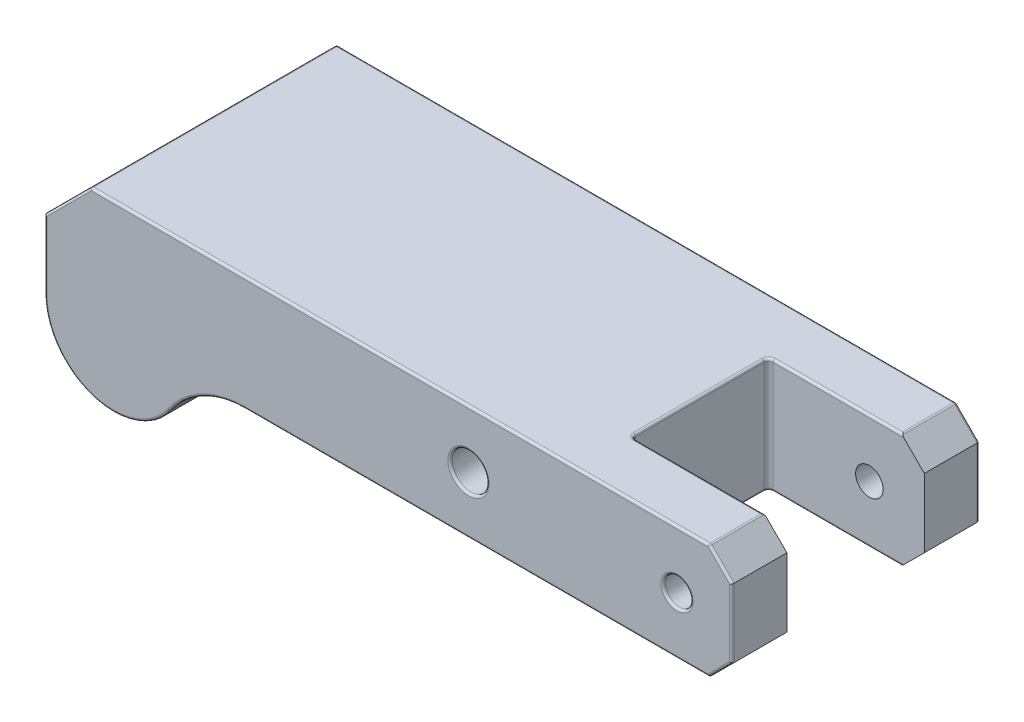
SolidWorks part; units mm, degrees
material "Plain Carbon Steel"
ref_plane "Front Plane" through (0, 0, 0) normal (0, 0, 1) x (1, 0, 0)
ref_plane "Top Plane" through (0, 0, 0) normal (0, 1, 0) x (1, 0, 0)
ref_plane "Right Plane" through (0, 0, 0) normal (1, 0, 0) x (0, 0, -1)
sketch "Arm Profile Sketch" plane through (0, 0, 0) normal (0, 0, 1) x (1, 0, 0)
  line L0 (0, 0) -> (-48.107, 0)
  line L1 (0, 0) -> (58.1702, 0)
  line L2 (58.1702, 0) -> (58.1702, 25)
  line L3 (58.1702, 25) -> (-91.8298, 25)
  line L4 (-91.8298, 25) -> (-91.8298, 0)
  arc A0 (-91.8298, 0) -> (-64.52, -8.5714) centre (-76.8298, 0) ccw
  arc A1 (-64.52, -8.5714) -> (-48.107, 0) centre (-48.107, -20) cw
  dimension "D1" = 30
  dimension "D3" = 20
  dimension "D4" = 91.8298
  dimension "D2" = 150
  dimension "D5" = 25
extrude "Arm Body 54mm" add sketch "Arm Profile Sketch" along normal mid plane 54
sketch "Fork Slot Sketch" plane through (0, 25, 0) normal (0, 1, 0) x (1, 0, 0)
  line L0 (58.1702, 15) -> (24.1702, 15)
  line L1 (58.1702, -27) -> (58.1702, 27) construction
  line L2 (24.1702, 15) -> (24.1702, -15)
  line L3 (24.1702, -15) -> (58.1702, -15)
  line L4 (58.1702, -15) -> (58.1702, 15)
  line L5 (58.1702, 27) -> (-91.8298, 27) construction
  line L6 (58.1702, -27) -> (-91.8298, -27) construction
  dimension "D1" = 12
  dimension "D2" = 12
  dimension "D3" = 34
extrude "Fork Slot 12mm" cut sketch "Fork Slot Sketch" against normal blind 54
chamfer "End Chamfer 5mm" distance 5 angle 45 4 edges at (58.1702, 0, -21) (58.1702, 0, 21) (58.1702, 25, -21) (58.1702, 25, 21)
chamfer "Corner Chamfer 10mm" distance 10 angle 45 1 edges at (-91.8298, 25, 0)
sketch "Pin Holes Sketch" plane through (0, 0, 27) normal (0, 0, 1) x (1, 0, 0)
  line L0 (58.1702, 5) -> (58.1702, 20) construction
  circle A0 centre (0.6702, 12.5) radius 4
  circle A1 centre (46.1702, 12.5) radius 3
  point P6 (58.1702, 12.5)
  dimension "D1" = 8
  dimension "D2" = 6
  dimension "D3" = 12
  dimension "D4" = 45.5
extrude "Pin Holes" cut sketch "Pin Holes Sketch" against normal blind 54
fillet "Slot Fillet R1" radius 1 2 edges at (24.1702, 12.5, -15) (24.1702, 12.5, 15)
fillet "Edge Fillet R0.5 A" radius 0.5 22 edges at (55.6702, 22.5, 27) (58.1702, 12.5, 27) (55.6702, 2.5, 27) (2.5316, 0, 27) (-57.3652, -2.2719, 27) (-81.3217, -14.3117, 27) (-91.8298, 7.5, 27) (-86.8298, 20, 27) (-14.3298, 25, 27) (49.1702, 12.5, 27) (4.6702, 12.5, 27) (-81.3217, -14.3117, -27) (-57.3652, -2.2719, -27) (2.5316, 0, -27) (55.6702, 2.5, -27) (58.1702, 12.5, -27) (55.6702, 22.5, -27) (-14.3298, 25, -27) (-86.8298, 20, -27) (-91.8298, 7.5, -27) (49.1702, 12.5, -27) (4.6702, 12.5, -27)
fillet "Edge Fillet R0.5 B" radius 0.5 21 edges at (53.1095, 0.1464, -26.8536) (53.1095, 0.1464, 26.8536) (53.1095, 24.8536, -26.8536) (53.1095, 24.8536, 26.8536) (-81.7692, 24.8536, -26.8536) (-81.7692, 24.8536, 26.8536) (39.1702, 0, 15) (24.4631, 0, 14.7071) (24.1702, 0, 0) (24.4631, 0, -14.7071) (39.1702, 0, -15) (53.1702, 0, -20.75) (53.1702, 0, 20.75) (53.1702, 25, -20.75) (39.1702, 25, -15) (24.4631, 25, -14.7071) (24.1702, 25, 0) (24.4631, 25, 14.7071) (39.1702, 25, 15) (53.1702, 25, 20.75) (-81.8298, 25, 0)
